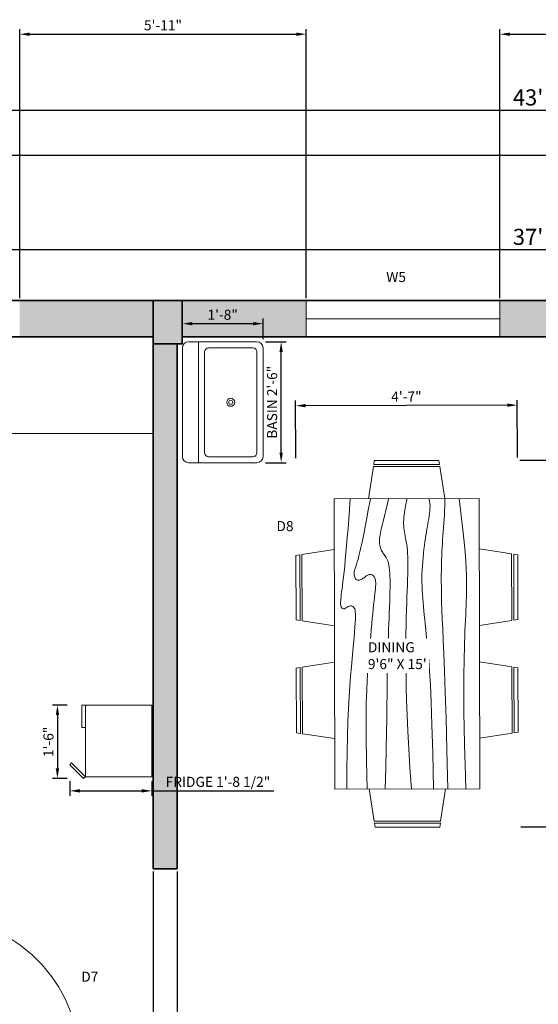
# Model space of a CAD drawing. Units: inches. Extents: x 5395 to 6469, y -203 to 448.
# Tile 4 of 7: x 5587 to 5715, y 204 to 448. Entities that reach past the tile are written whole.
import ezdxf

# ---------------------------------------------------------------- set-up
doc = ezdxf.new("R2010")
doc.units = ezdxf.units.IN
for name, color, linetype, lineweight in [('A-ANNO-DIMS', 2, 'Continuous', 18), ('A-ANNO-TEXT', 6, 'Continuous', 18), ('A-AREA-IDEN', 6, 'Continuous', 18), ('A-COLS', 7, 'Continuous', 35), ('A-COLS-PATT', 2, 'Continuous', 13), ('A-EQPM', 70, 'Continuous', 18), ('A-FLOR-CASE', 32, 'Continuous', 18), ('A-FLOR-FIXT', 70, 'Continuous', 18), ('A-GLAZ', 4, 'Continuous', 18), ('A-WALL', 7, 'Continuous', 35), ('A-WALL-PATT', 11, 'Continuous', 9), ('C-PROP', 7, 'Continuous', 25), ('door', 240, 'Continuous', 18), ('furniture', 70, 'Continuous', 18)]:
    doc.layers.add(name, color=color, linetype=linetype, lineweight=lineweight)
doc.styles.get("Standard").update_dxf_attribs({"font": 'arial.ttf'})
doc.dimstyles.new('ISO-25', dxfattribs={"dimtxt": 2.5, "dimasz": 2.5, "dimexe": 1.25, "dimexo": 0.625, "dimtad": 1, "dimdec": 1, "dimlunit": 3, "dimtxsty": 'Standard', "dimcen": 2.5, "dimadec": 0, "dimazin": 0, "dimtfac": 1, "dimtdec": 1, "dimtmove": 0, "dimatfit": 3, "dimfxl": 1, "dimarcsym": 0})

# ---------------------------------------------------------------- blocks, each defined once
blk = doc.blocks.new('*U4')
for p, q in [((0, 0), (0, 5)), ((30, 0), (30, 5))]:
    blk.add_line(p, q)
blk.add_lwpolyline([(0, 0), (0, -30), (1.75, -30), (1.75, 0)], close=True)
blk.add_arc((0, 0), 30, 270, 0)
blk = doc.blocks.new('Dining Set - 36 x 72 in.')
for p, q in [((-22, 27.5), (-22.1562, 26.50042)), ((-22, 27.5), (-6, 27.5)), ((-5.8437, 26.49966), (-6, 27.5)), ((6, 27.5), (5.8438, 26.50042)), ((6, 27.5), (22, 27.5)), ((22.1563, 26.49966), (22, 27.5)), ((-22.2343, 26.00059), (-23.4847, 17.99762)), ((-22.2304, 26), (-5.7608, 26)), ((-5.8416, 26.5), (-22.1534, 26.5)), ((-4.5152, 17.99762), (-5.7655, 25.99926)), ((5.7657, 26.00059), (4.5153, 17.99762)), ((5.7696, 26), (22.2392, 26)), ((22.1584, 26.5), (5.8466, 26.5)), ((23.4848, 17.99762), (22.2345, 25.99926)), ((36, 18), (-36, 18)), ((-36, 18), (-36, -18)), ((36, -18), (36, 18)), ((-45.5, 8), (-44.5004, 8.15617)), ((-45.5, 8), (-45.5, -8)), ((-44.5, -8.15843), (-44.5, 8.15338)), ((-44.0006, 8.23428), (-35.9976, 9.48474)), ((-44, 8.23041), (-44, -8.23915)), ((44.0006, 8.23428), (35.9976, 9.48474)), ((44, 8.23041), (44, -8.23915)), ((44.5, -8.15843), (44.5, 8.15338)), ((45.5, 8), (44.5005, 8.15617)), ((45.5, 8), (45.5, -8)), ((-44.4997, -8.15631), (-45.5, -8)), ((-35.9976, -9.48476), (-43.9993, -8.2345)), ((35.9976, -9.48476), (43.9993, -8.2345)), ((44.4997, -8.15631), (45.5, -8)), ((-36, -18), (36, -18)), ((-22.2343, -26.0006), (-23.4847, -17.99762)), ((-4.5152, -17.99762), (-5.7655, -25.99928)), ((5.7657, -26.0006), (4.5153, -17.99762)), ((23.4848, -17.99762), (22.2345, -25.99928)), ((-22.2304, -26), (-5.7608, -26)), ((-22, -27.5), (-22.1562, -26.50044)), ((-5.8416, -26.5), (-22.1534, -26.5)), ((-5.8437, -26.49967), (-6, -27.5)), ((5.7696, -26), (22.2392, -26)), ((6, -27.5), (5.8438, -26.50044)), ((22.1584, -26.5), (5.8466, -26.5)), ((22.1563, -26.49967), (22, -27.5)), ((-22, -27.5), (-6, -27.5)), ((6, -27.5), (22, -27.5))]:
    blk.add_line(p, q)
for points in [[(-36, 15), (-31.1772, 14.97754), (-26.8079, 14.91406), (-22.8538, 14.81543), (-19.276, 14.6875), (-16.0362, 14.53613), (-13.0957, 14.36718), (-10.4159, 14.18652), (-7.9583, 14), (-5.6904, 13.81315), (-3.6035, 13.63021), (-1.6954, 13.45508), (0.0365, 13.29166), (1.5945, 13.14388), (2.9811, 13.01562), (4.1988, 12.9108), (5.25, 12.83333), (6.1393, 12.78613), (6.8802, 12.76823), (7.4883, 12.77767), (7.9792, 12.8125), (8.3685, 12.87077), (8.6719, 12.95052), (8.9049, 13.0498), (9.0833, 13.16666), (9.2205, 13.29899), (9.3216, 13.44401), (9.3895, 13.59879), (9.4271, 13.76041), (9.4373, 13.92594), (9.4232, 14.09245), (9.3875, 14.257), (9.3333, 14.41666), (9.2638, 14.56917), (9.1836, 14.71484), (9.0975, 14.85465), (9.0104, 14.98958), (8.9272, 15.1206), (8.8529, 15.2487), (8.7922, 15.37483), (8.75, 15.5), (8.7305, 15.62467), (8.7344, 15.74739), (8.7617, 15.86621), (8.8125, 15.97916), (8.8867, 16.08431), (8.9844, 16.17968), (9.1055, 16.26334), (9.25, 16.33333), (9.4189, 16.38802), (9.6172, 16.42708), (9.8506, 16.45052), (10.125, 16.45833), (10.4463, 16.45052), (10.8203, 16.42708), (11.2529, 16.38802), (11.75, 16.33333), (12.3184, 16.26318), (12.9694, 16.17838), (13.7151, 16.07991), (14.5677, 15.96875), (15.5395, 15.84586), (16.6426, 15.71224), (17.8893, 15.56884), (19.2917, 15.41666), (20.859, 15.25667), (22.5879, 15.08984), (24.4721, 14.91715), (26.5052, 14.73958), (28.6809, 14.5581), (30.9929, 14.3737), (33.4347, 14.18733), (36, 14)], [(-36, 10), (-28.9766, 10.14274), (-23.1725, 10.20442), (-18.4241, 10.19775), (-14.5677, 10.13541), (-11.4399, 10.03011), (-8.877, 9.89453), (-6.7154, 9.74137), (-4.7917, 9.58333), (-2.9698, 9.43082), (-1.2246, 9.28515), (0.4415, 9.14534), (2.026, 9.01041), (3.5266, 8.87939), (4.9408, 8.7513), (6.266, 8.62516), (7.5, 8.5), (8.6411, 8.37549), (9.6914, 8.2539), (10.6538, 8.13818), (11.5312, 8.03125), (12.3267, 7.93603), (13.043, 7.85547), (13.6831, 7.79248), (14.25, 7.75), (14.7471, 7.7303), (15.1797, 7.73307), (15.5537, 7.75732), (15.875, 7.80208), (16.1494, 7.86637), (16.3828, 7.94922), (16.5811, 8.04964), (16.75, 8.16666), (16.8944, 8.29915), (17.0143, 8.44531), (17.1089, 8.60319), (17.1771, 8.77083), (17.218, 8.94629), (17.2305, 9.1276), (17.2137, 9.31282), (17.1667, 9.5), (17.0895, 9.6875), (16.987, 9.875), (16.8649, 10.0625), (16.7292, 10.25), (16.5856, 10.4375), (16.4401, 10.625), (16.2985, 10.8125), (16.1667, 11), (16.05, 11.18733), (15.9518, 11.3737), (15.8752, 11.5581), (15.8229, 11.73958), (15.798, 11.91715), (15.8034, 12.08984), (15.842, 12.25667), (15.9167, 12.41666), (16.0295, 12.56836), (16.1784, 12.70833), (16.3605, 12.83268), (16.5729, 12.9375), (16.8127, 13.01888), (17.0768, 13.07291), (17.3625, 13.0957), (17.6667, 13.08333), (17.9894, 13.03312), (18.3418, 12.94726), (18.7382, 12.82918), (19.1927, 12.68229), (19.7195, 12.51001), (20.3327, 12.31575), (21.0465, 12.10294), (21.875, 11.875), (22.8357, 11.63354), (23.959, 11.37304), (25.2786, 11.08618), (26.8282, 10.76562), (28.6414, 10.40405), (30.752, 9.99414), (33.1936, 9.52856), (36, 9)], [(-36, 5.5), (-30.7157, 5.3348), (-26.069, 5.20963), (-21.9946, 5.11767), (-18.4271, 5.05208), (-15.3009, 5.00602), (-12.5508, 4.97265), (-10.1112, 4.94515), (-7.9167, 4.91666), (-5.909, 4.88167), (-4.0586, 4.83984), (-2.3429, 4.79215), (-0.7396, 4.73958), (0.7739, 4.6831), (2.22, 4.6237), (3.6213, 4.56233), (5, 4.5), (6.373, 4.43782), (7.7344, 4.3776), (9.0723, 4.32129), (10.375, 4.27083), (11.6309, 4.22819), (12.8281, 4.19531), (13.9551, 4.17415), (15, 4.16666), (15.954, 4.17448), (16.819, 4.19791), (17.6001, 4.23698), (18.3021, 4.29166), (18.9299, 4.36198), (19.4883, 4.44791), (19.9823, 4.54948), (20.4167, 4.66666), (20.7969, 4.79899), (21.1302, 4.94401), (21.4245, 5.09879), (21.6875, 5.26041), (21.9271, 5.42594), (22.1511, 5.59245), (22.3672, 5.757), (22.5834, 5.91666), (22.8065, 6.06868), (23.0404, 6.21093), (23.2879, 6.34147), (23.5521, 6.45833), (23.8358, 6.55957), (24.142, 6.64323), (24.4735, 6.70735), (24.8334, 6.75), (25.2235, 6.76969), (25.642, 6.76692), (26.0858, 6.74267), (26.5521, 6.69791), (27.0379, 6.63362), (27.5404, 6.55078), (28.0565, 6.45036), (28.5834, 6.33333), (29.1242, 6.19987), (29.7071, 6.04687), (30.3661, 5.87044), (31.1354, 5.66666), (32.0493, 5.43164), (33.142, 5.16146), (34.4475, 4.85221), (36, 4.5)], [(-36, -1), (-30.7915, -0.6591), (-26.0195, -0.38216), (-21.6519, -0.16284), (-17.6563, 0.00521), (-14.0005, 0.12833), (-10.6523, 0.21289), (-7.5796, 0.26522), (-4.75, 0.29166), (-2.134, 0.29793), (0.2878, 0.28711), (2.5317, 0.26163), (4.6146, 0.22396), (6.5529, 0.17651), (8.3633, 0.12174), (10.0623, 0.06209), (11.6667, 0), (13.1899, -0.06201), (14.6341, -0.1211), (15.9982, -0.17432), (17.2813, -0.21875), (18.4823, -0.25147), (19.6003, -0.26953), (20.6343, -0.27002), (21.5834, -0.25), (22.4481, -0.20768), (23.2357, -0.14584), (23.9549, -0.06836), (24.6146, 0.02083), (25.2235, 0.11784), (25.7904, 0.21875), (26.3241, 0.31966), (26.8334, 0.41666), (27.3265, 0.50618), (27.8099, 0.58593), (28.2894, 0.65397), (28.7709, 0.70833), (29.2601, 0.74707), (29.763, 0.76823), (30.2855, 0.76985), (30.8334, 0.75), (31.4088, 0.70784), (31.9994, 0.64713), (32.589, 0.57275), (33.1615, 0.48958), (33.7008, 0.4025), (34.1908, 0.3164), (34.6153, 0.23616), (34.9584, 0.16666), (35.2099, 0.11165), (35.3848, 0.07031), (35.504, 0.04069), (35.5886, 0.02083), (35.6594, 0.00879), (35.7377, 0.0026), (35.8442, 0.00032), (36, 0)], [(-36, -6.5), (-27.1843, -6.31267), (-20.084, -6.1263), (-14.469, -5.9419), (-10.1094, -5.76042), (-6.7752, -5.58285), (-4.2363, -5.41016), (-2.2629, -5.24333), (-0.625, -5.08334), (0.8708, -4.93099), (2.2715, -4.78646), (3.5872, -4.64974), (4.8281, -4.52084), (6.0046, -4.39974), (7.127, -4.28646), (8.2053, -4.18099), (9.25, -4.08334), (10.2705, -3.99382), (11.2734, -3.91407), (12.2647, -3.84603), (13.25, -3.79167), (14.2354, -3.75293), (15.2266, -3.73177), (16.2295, -3.73015), (17.25, -3.75), (18.2912, -3.79248), (19.3451, -3.85547), (20.4009, -3.93604), (21.4479, -4.03125), (22.4754, -4.13819), (23.4727, -4.25391), (24.4289, -4.37549), (25.3334, -4.5), (26.1785, -4.62492), (26.9694, -4.74935), (27.7145, -4.87281), (28.4219, -4.99479), (29.1, -5.11483), (29.7572, -5.23242), (30.4016, -5.34709), (31.0417, -5.45834), (31.6837, -5.56437), (32.3262, -5.65821), (32.9658, -5.73153), (33.599, -5.77604), (34.2224, -5.78345), (34.8327, -5.74545), (35.4264, -5.65373), (36, -5.5)], [(-36, -10), (-26.4022, -9.81299), (-18.4675, -9.62891), (-11.9839, -9.45069), (-6.7396, -9.28125), (-2.5226, -9.12354), (0.8789, -8.98047), (3.6769, -8.85498), (6.0833, -8.75), (8.2767, -8.66765), (10.3021, -8.60677), (12.1712, -8.56543), (13.8958, -8.54167), (15.4876, -8.53353), (16.9583, -8.53907), (18.3197, -8.55632), (19.5834, -8.58334), (20.7616, -8.61841), (21.8685, -8.66081), (22.9188, -8.71004), (23.9271, -8.76563), (24.9081, -8.82707), (25.8763, -8.89388), (26.8465, -8.96558), (27.8334, -9.04167), (28.8474, -9.12118), (29.8828, -9.20117), (30.93, -9.27824), (31.9792, -9.34896), (33.0205, -9.40991), (34.0443, -9.45768), (35.0407, -9.48885), (36, -9.5)], [(-36, -14.5), (-30.0881, -14.33513), (-25.0332, -14.21224), (-20.7312, -14.12647), (-17.0781, -14.07292), (-13.97, -14.04671), (-11.3027, -14.04297), (-8.9724, -14.05681), (-6.875, -14.08334), (-4.9224, -14.11833), (-3.0905, -14.16016), (-1.3709, -14.20785), (0.2448, -14.26042), (1.7647, -14.3169), (3.1973, -14.3763), (4.5507, -14.43767), (5.8333, -14.5), (7.0554, -14.5621), (8.235, -14.62175), (9.3922, -14.67652), (10.5469, -14.72396), (11.7192, -14.76164), (12.929, -14.78711), (14.1965, -14.79794), (15.5417, -14.79167), (16.9933, -14.76424), (18.6152, -14.70508), (20.4804, -14.60197), (22.6615, -14.44271), (25.2312, -14.21509), (28.2624, -13.9069), (31.8277, -13.50594), (36, -13)]]:
    blk.add_lwpolyline(points)
blk = doc.blocks.new('Sink-single - 30 in top')
blk.add_line((-15, -3.999996), (15, -3.999996))
for points in [[(-13.5, 0), (13.5, 0)], [(-15, -18.499996), (-15, -1.5)], [(15, -1.5), (15, -18.499996)], [(-13.5, -17.499996), (-13.5, -6.499996)], [(-12.5, -5.499996), (12.5, -5.499996)], [(13.5, -6.499996), (13.5, -17.499996)], [(12.5, -18.499996), (-12.5, -18.499996)], [(13.5, -19.999996), (-13.5, -19.999996)]]:
    blk.add_lwpolyline(points)
for radius in [1, 0.5]:
    blk.add_circle((0, -11.999996), radius)
for centre, radius, start, end in [((-13.5, -1.5), 1.5, 90, 180), ((13.5, -1.5), 1.5, 0, 90), ((-12.5, -6.499996), 1, 90, 180), ((12.5, -6.499996), 1, 0, 90), ((-13.5, -18.499996), 1.5, 180, 270), ((-12.5, -17.499996), 1, 180, 270), ((12.5, -17.499996), 1, 270, 0), ((13.5, -18.499996), 1.5, 270, 0)]:
    blk.add_arc(centre, radius, start, end)
blk = doc.blocks.new('FRIDGE')
for points in [[(0, 16.47), (17.77, 16.47), (17.77, 0), (0, 0)], [(0, 0), (5.53, 0), (5.53, -0.88), (0, -0.88)], [(18.23, -0.47), (17.77, 0), (14.32, -3.43), (14.79, -3.9)]]:
    blk.add_lwpolyline(points, close=True)
blk = doc.blocks.new('*D17')
at = {"layer": 'A-ANNO-DIMS', "color": 0, "lineweight": -2, "transparency": 16777216}
for p, q in [((5490.94, 378.93), (5490.94, 392.2)), ((5493.44, 390.95), (5932.44, 390.95)), ((5934.94, 378.93), (5934.94, 392.2))]:
    blk.add_line(p, q, dxfattribs=at)
at = {"layer": 'A-ANNO-DIMS', "color": 0, "transparency": 16777216}
for points in [[(5493.44, 391.36), (5493.44, 390.53), (5490.94, 390.95)], [(5932.44, 391.36), (5932.44, 390.53), (5934.94, 390.95)]]:
    blk.add_solid(points, dxfattribs=at)
at = {"layer": 'Defpoints', "color": 0, "transparency": 16777216}
for p in [(5934.94, 390.95), (5490.94, 378.31), (5934.94, 378.31)]:
    blk.add_point(p, dxfattribs=at)
at = {"layer": 'A-ANNO-DIMS', "color": 0, "transparency": 16777216, "insert": (5712.94, 393.61), "char_height": 4, "attachment_point": 5}
blk.add_mtext("37'", dxfattribs=at)
blk = doc.blocks.new('*D18')
at = {"layer": 'A-ANNO-DIMS', "color": 0, "lineweight": -2, "transparency": 16777216}
for p, q in [((5454.94, 414.93), (5454.94, 426.78)), ((5457.44, 425.53), (5968.44, 425.53)), ((5970.94, 414.93), (5970.94, 426.78))]:
    blk.add_line(p, q, dxfattribs=at)
at = {"layer": 'A-ANNO-DIMS', "color": 0, "transparency": 16777216}
for points in [[(5457.44, 425.95), (5457.44, 425.12), (5454.94, 425.53)], [(5968.44, 425.95), (5968.44, 425.12), (5970.94, 425.53)]]:
    blk.add_solid(points, dxfattribs=at)
at = {"layer": 'Defpoints', "color": 0, "transparency": 16777216}
for p in [(5970.94, 425.53), (5454.94, 414.31), (5970.94, 414.31)]:
    blk.add_point(p, dxfattribs=at)
at = {"layer": 'A-ANNO-DIMS', "color": 0, "transparency": 16777216, "insert": (5712.94, 428.2), "char_height": 4, "attachment_point": 5}
blk.add_mtext("43'", dxfattribs=at)
blk = doc.blocks.new('WINDOW-48IN')
for p, q in [((0, 0), (0, 9)), ((48, 0), (48, 9)), ((0, 4.5), (48, 4.5))]:
    blk.add_line(p, q)
blk = doc.blocks.new('*D51')
at = {"layer": 'A-ANNO-DIMS', "color": 0, "lineweight": -2, "transparency": 16777216}
for p, q in [((5710.93, 338.72), (5725.21, 338.76)), ((5724.17, 250.25), (5723.96, 336.25)), ((5711.15, 247.72), (5725.43, 247.76))]:
    blk.add_line(p, q, dxfattribs=at)
at = {"layer": 'A-ANNO-DIMS', "color": 0, "transparency": 16777216}
for points in [[(5724.38, 336.25), (5723.55, 336.25), (5723.96, 338.75)], [(5724.59, 250.25), (5723.75, 250.25), (5724.18, 247.75)]]:
    blk.add_solid(points, dxfattribs=at)
at = {"layer": 'Defpoints', "color": 0, "transparency": 16777216}
for p in [(5710.31, 338.72), (5723.96, 338.75), (5710.53, 247.72)]:
    blk.add_point(p, dxfattribs=at)
at = {"layer": 'A-ANNO-DIMS', "color": 0, "transparency": 16777216, "insert": (5725.98, 293.26), "char_height": 2.5, "attachment_point": 5, "rotation": 270.1373}
blk.add_mtext('DINING SET 7\'-7"', dxfattribs=at)
blk = doc.blocks.new('*D52')
at = {"layer": 'A-ANNO-DIMS', "color": 0, "lineweight": -2, "transparency": 16777216}
for p, q in [((5655.31, 339.21), (5655.27, 353.49)), ((5707.77, 352.36), (5657.78, 352.24)), ((5710.31, 339.34), (5710.27, 353.62))]:
    blk.add_line(p, q, dxfattribs=at)
at = {"layer": 'A-ANNO-DIMS', "color": 0, "transparency": 16777216}
for points in [[(5657.77, 352.66), (5657.78, 351.83), (5655.28, 352.24)], [(5707.77, 352.78), (5707.78, 351.95), (5710.27, 352.37)]]:
    blk.add_solid(points, dxfattribs=at)
at = {"layer": 'Defpoints', "color": 0, "transparency": 16777216}
for p in [(5655.28, 352.24), (5655.31, 338.59), (5710.31, 338.72)]:
    blk.add_point(p, dxfattribs=at)
at = {"layer": 'A-ANNO-DIMS', "color": 0, "transparency": 16777216, "insert": (5682.77, 354.18), "char_height": 2.5, "attachment_point": 5, "rotation": 0.1373}
blk.add_mtext('4\'-7"', dxfattribs=at)
blk = doc.blocks.new('*D53')
at = {"layer": 'A-ANNO-DIMS', "color": 0, "lineweight": -2, "transparency": 16777216}
for p, q in [((5647.83, 368.08), (5652.96, 368.08)), ((5651.71, 340.58), (5651.71, 365.58)), ((5647.83, 338.08), (5652.96, 338.08))]:
    blk.add_line(p, q, dxfattribs=at)
at = {"layer": 'A-ANNO-DIMS', "color": 0, "transparency": 16777216}
for points in [[(5651.29, 365.58), (5652.12, 365.58), (5651.71, 368.08)], [(5651.29, 340.58), (5652.12, 340.58), (5651.71, 338.08)]]:
    blk.add_solid(points, dxfattribs=at)
at = {"layer": 'Defpoints', "color": 0, "transparency": 16777216}
for p in [(5647.21, 368.08), (5651.71, 368.08), (5647.21, 338.08)]:
    blk.add_point(p, dxfattribs=at)
at = {"layer": 'A-ANNO-DIMS', "color": 0, "transparency": 16777216, "insert": (5649.79, 353.08), "char_height": 2.5, "attachment_point": 5, "rotation": 90}
blk.add_mtext('BASIN 2\'-6"', dxfattribs=at)
blk = doc.blocks.new('*D54')
at = {"layer": 'A-ANNO-DIMS', "color": 0, "lineweight": -2, "transparency": 16777216}
for p, q in [((5627.21, 368.71), (5627.21, 373.83)), ((5647.21, 368.71), (5647.21, 373.83)), ((5644.71, 372.58), (5629.71, 372.58))]:
    blk.add_line(p, q, dxfattribs=at)
at = {"layer": 'A-ANNO-DIMS', "color": 0, "transparency": 16777216}
for points in [[(5629.71, 373), (5629.71, 372.17), (5627.21, 372.58)], [(5644.71, 373), (5644.71, 372.17), (5647.21, 372.58)]]:
    blk.add_solid(points, dxfattribs=at)
at = {"layer": 'Defpoints', "color": 0, "transparency": 16777216}
for p in [(5627.21, 372.58), (5627.21, 368.08), (5647.21, 368.08)]:
    blk.add_point(p, dxfattribs=at)
at = {"layer": 'A-ANNO-DIMS', "color": 0, "transparency": 16777216, "insert": (5637.21, 374.48), "char_height": 2.5, "attachment_point": 5}
blk.add_mtext('1\'-8"', dxfattribs=at)
blk = doc.blocks.new('*D55')
at = {"layer": 'A-ANNO-DIMS', "color": 0, "lineweight": -2, "transparency": 16777216}
for p, q in [((5599.29, 259.09), (5599.29, 255.41)), ((5619.66, 259.09), (5619.66, 255.41)), ((5601.79, 256.66), (5617.16, 256.66)), ((5619.66, 256.66), (5649.9, 256.66))]:
    blk.add_line(p, q, dxfattribs=at)
at = {"layer": 'A-ANNO-DIMS', "color": 0, "transparency": 16777216}
for points in [[(5601.79, 257.08), (5601.79, 256.25), (5599.29, 256.66)], [(5617.16, 257.08), (5617.16, 256.25), (5619.66, 256.66)]]:
    blk.add_solid(points, dxfattribs=at)
at = {"layer": 'Defpoints', "color": 0, "transparency": 16777216}
for p in [(5599.29, 259.72), (5619.66, 259.72), (5619.66, 256.66)]:
    blk.add_point(p, dxfattribs=at)
at = {"layer": 'A-ANNO-DIMS', "color": 0, "transparency": 16777216, "insert": (5636.03, 258.58), "char_height": 2.5, "attachment_point": 5}
blk.add_mtext('FRIDGE 1\'-8 1/2"', dxfattribs=at)
blk = doc.blocks.new('*D56')
at = {"layer": 'A-ANNO-DIMS', "color": 0, "lineweight": -2, "transparency": 16777216}
for p, q in [((5598.66, 277.95), (5594.98, 277.95)), ((5596.23, 275.45), (5596.23, 262.22)), ((5598.66, 259.72), (5594.98, 259.72))]:
    blk.add_line(p, q, dxfattribs=at)
at = {"layer": 'A-ANNO-DIMS', "color": 0, "transparency": 16777216}
for points in [[(5595.82, 275.45), (5596.65, 275.45), (5596.23, 277.95)], [(5595.82, 262.22), (5596.65, 262.22), (5596.23, 259.72)]]:
    blk.add_solid(points, dxfattribs=at)
at = {"layer": 'Defpoints', "color": 0, "transparency": 16777216}
for p in [(5599.29, 277.95), (5596.23, 259.72), (5599.29, 259.72)]:
    blk.add_point(p, dxfattribs=at)
at = {"layer": 'A-ANNO-DIMS', "color": 0, "transparency": 16777216, "insert": (5594.33, 268.83), "char_height": 2.5, "attachment_point": 5, "rotation": 90}
blk.add_mtext('1\'-6"', dxfattribs=at)
blk = doc.blocks.new('*D62')
at = {"layer": 'A-ANNO-DIMS', "color": 0, "lineweight": -2, "transparency": 16777216}
for p, q in [((5586.88, 378.93), (5586.88, 445.66)), ((5657.93, 378.93), (5657.93, 445.66)), ((5589.38, 444.41), (5655.43, 444.41))]:
    blk.add_line(p, q, dxfattribs=at)
at = {"layer": 'A-ANNO-DIMS', "color": 0, "transparency": 16777216}
for points in [[(5589.38, 444.82), (5589.38, 443.99), (5586.88, 444.41)], [(5655.43, 444.82), (5655.43, 443.99), (5657.93, 444.41)]]:
    blk.add_solid(points, dxfattribs=at)
at = {"layer": 'Defpoints', "color": 0, "transparency": 16777216}
for p in [(5657.93, 444.41), (5586.88, 378.31), (5657.93, 378.31)]:
    blk.add_point(p, dxfattribs=at)
at = {"layer": 'A-ANNO-DIMS', "color": 0, "transparency": 16777216, "insert": (5622.4, 446.31), "char_height": 2.5, "attachment_point": 5}
blk.add_mtext('5\'-11"', dxfattribs=at)
blk = doc.blocks.new('*D63')
at = {"layer": 'A-ANNO-DIMS', "color": 0, "lineweight": -2, "transparency": 16777216}
for p, q in [((5705.93, 378.93), (5705.93, 445.66)), ((5812.1, 378.93), (5812.1, 445.66)), ((5708.43, 444.41), (5809.6, 444.41))]:
    blk.add_line(p, q, dxfattribs=at)
at = {"layer": 'A-ANNO-DIMS', "color": 0, "transparency": 16777216}
for points in [[(5708.43, 444.82), (5708.43, 443.99), (5705.93, 444.41)], [(5809.6, 444.82), (5809.6, 443.99), (5812.1, 444.41)]]:
    blk.add_solid(points, dxfattribs=at)
at = {"layer": 'Defpoints', "color": 0, "transparency": 16777216}
for p in [(5812.1, 444.41), (5705.93, 378.31), (5812.1, 378.31)]:
    blk.add_point(p, dxfattribs=at)
at = {"layer": 'A-ANNO-DIMS', "color": 0, "transparency": 16777216, "insert": (5759.01, 446.31), "char_height": 2.5, "attachment_point": 5}
blk.add_mtext('8\'-10"', dxfattribs=at)
blk = doc.blocks.new('*D72')
at = {"layer": 'A-ANNO-DIMS', "color": 0, "lineweight": -2, "transparency": 16777216}
for p, q in [((5619.94, 236.68), (5619.94, -186.04)), ((5625.94, 236.68), (5625.94, -186.04)), ((5617.44, -184.79), (5614.94, -184.79)), ((5619.94, -184.79), (5625.94, -184.79)), ((5628.44, -184.79), (5638.83, -184.79))]:
    blk.add_line(p, q, dxfattribs=at)
at = {"layer": 'A-ANNO-DIMS', "color": 0, "transparency": 16777216}
for points in [[(5617.44, -184.38), (5617.44, -185.21), (5619.94, -184.79)], [(5628.44, -184.38), (5628.44, -185.21), (5625.94, -184.79)]]:
    blk.add_solid(points, dxfattribs=at)
at = {"layer": 'Defpoints', "color": 0, "transparency": 16777216}
for p in [(5619.94, 237.31), (5625.94, 237.31), (5625.94, -184.79)]:
    blk.add_point(p, dxfattribs=at)
at = {"layer": 'A-ANNO-DIMS', "color": 0, "transparency": 16777216, "insert": (5634.88, -182.89), "char_height": 2.5, "attachment_point": 5}
blk.add_mtext('0\'-6"', dxfattribs=at)

msp = doc.modelspace()

# ---------------------------------------------------------------- hatches: boundary and pattern name
at = {"layer": 'A-COLS-PATT'}
h = msp.add_hatch(color=256, dxfattribs=at)
h.dxf.hatch_style = 1
h.paths.add_polyline_path([(5627.19, 378.31), (5619.94, 378.31), (5619.94, 369.31), (5619.94, 367.55), (5627.19, 367.55), (5627.19, 369.31)])
h.paths.add_polyline_path([(5753.55, 378.31), (5739.94, 378.31), (5739.94, 369.31), (5753.55, 369.31)])
h.paths.add_polyline_path([(5934.94, 378.31), (5923.7, 378.31), (5923.7, 369.31), (5925.94, 369.31), (5934.94, 369.31)])
at = {"layer": 'A-WALL-PATT'}
h = msp.add_hatch(color=256, dxfattribs=at)
h.dxf.hatch_style = 1
h.paths.add_polyline_path([(5538.88, 378.31), (5499.94, 378.31), (5499.94, 369.31), (5538.88, 369.31)])
h.paths.add_polyline_path([(5499.94, 276.14), (5490.94, 276.14), (5490.94, 227.71), (5499.94, 227.71), (5499.94, 237.31)])
h.paths.add_polyline_path([(5565.94, 243.31), (5499.94, 243.31), (5499.94, 237.31), (5559.94, 237.31), (5559.94, 225.31), (5565.94, 225.31)])
h.paths.add_polyline_path([(5625.94, 367.55), (5619.94, 367.55), (5619.94, 237.31), (5625.94, 237.31)])
h.paths.add_polyline_path([(5745.94, 369.31), (5739.94, 369.31), (5739.94, 237.31), (5745.94, 237.31)])
h.paths.add_polyline_path([(5745.94, 192.25), (5739.94, 192.25), (5739.94, 190.23), (5745.94, 190.23)])
h.paths.add_polyline_path([(5745.94, 180.33), (5739.94, 180.33), (5739.94, 47.04), (5745.94, 47.04)])
h.paths.add_polyline_path([(5877.94, 183.31), (5884.03, 183.31), (5884.03, 189.31), (5747.34, 189.31), (5747.34, 183.31), (5871.94, 183.31), (5871.94, 82.27), (5877.94, 82.27), (5877.94, 90.31), (5925.94, 90.31), (5925.94, 96.31), (5877.94, 96.31)])
h.paths.add_polyline_path([(5934.94, 128.85), (5925.94, 128.85), (5925.94, 55.61), (5934.94, 55.61)])
h.paths.add_polyline_path([(5934.94, 181.4), (5925.94, 181.4), (5925.94, 152.85), (5934.94, 152.85)])
h.paths.add_polyline_path([(5925.94, 189.31), (5914.03, 189.31), (5914.03, 183.31), (5925.94, 183.31)], flags=17)
h.paths.add_polyline_path([(5934.94, 369.31), (5925.94, 369.31), (5925.94, 237.31), (5934.94, 237.31)])
h.paths.add_polyline_path([(5657.93, 378.31), (5627.19, 378.31), (5627.19, 369.31), (5657.93, 369.31)])
h.paths.add_polyline_path([(5619.94, 378.31), (5586.88, 378.31), (5586.88, 369.31), (5619.94, 369.31)])
h.paths.add_polyline_path([(5739.94, 378.31), (5705.93, 378.31), (5705.93, 369.31), (5739.94, 369.31)])
h.paths.add_polyline_path([(5812.1, 378.31), (5753.55, 378.31), (5753.55, 369.31), (5812.1, 369.31)])
h.paths.add_polyline_path([(5923.7, 378.31), (5860.1, 378.31), (5860.1, 369.31), (5923.7, 369.31)])
h.paths.add_polyline_path([(5499.94, 203.71), (5490.94, 203.71), (5490.94, 189.31), (5499.94, 189.31)])
h.paths.add_polyline_path([(5612.93, 189.31), (5499.94, 189.31), (5499.94, 183.31), (5612.93, 183.31)])
h.paths.add_polyline_path([(5499.94, 178.42), (5490.94, 178.42), (5490.94, 132.59), (5499.94, 132.59)])
h.paths.add_polyline_path([(5499.94, 84.59), (5490.94, 84.59), (5490.94, 47.04), (5499.94, 47.04)])
h.paths.add_polyline_path([(5499.94, 11.04), (5490.94, 11.04), (5490.94, 3.31), (5499.94, 3.31)])
h.paths.add_polyline_path([(5532.25, 3.31), (5502.78, 3.31), (5502.78, -5.69), (5532.25, -5.69)])
h.paths.add_polyline_path([(5601.84, 3.31), (5580.25, 3.31), (5580.25, -5.69), (5601.84, -5.69)])
h.paths.add_polyline_path([(5625.94, 3.31), (5614.13, 3.31), (5614.13, -5.69), (5625.94, -5.69)])
h.paths.add_polyline_path([(5787.9, 3.31), (5748.46, 3.31), (5748.46, -5.69), (5787.9, -5.69)])
h.paths.add_polyline_path([(5737.31, 3.31), (5697.94, 3.31), (5697.94, -5.69), (5737.31, -5.69)])
h.paths.add_polyline_path([(5745.94, 11.04), (5739.94, 11.04), (5739.94, 3.31), (5745.94, 3.31)])
h.paths.add_polyline_path([(5922.21, 3.31), (5877.94, 3.31), (5877.94, 46.27), (5871.94, 46.27), (5871.94, 3.31), (5835.9, 3.31), (5835.9, -5.69), (5922.21, -5.69)])
h.paths.add_polyline_path([(5934.94, 31.61), (5925.94, 31.61), (5925.94, 3.31), (5934.94, 3.31)])

# ---------------------------------------------------------------- linework, layer by layer
at = {"layer": 'A-COLS'}
for p, q in [((5619.94, 369.31), (5619.94, 378.31)), ((5627.19, 369.31), (5627.19, 378.31)), ((5627.19, 369.31), (5627.19, 367.55)), ((5619.94, 367.55), (5627.19, 367.55))]:
    msp.add_line(p, q, dxfattribs=at)
at = {"layer": 'A-FLOR-CASE'}
for points in [[(5499.94, 243.31), (5499.94, 369.31), (5619.94, 369.31)], [(5523.94, 243.31), (5523.94, 345.31), (5619.94, 345.31)]]:
    msp.add_lwpolyline(points, dxfattribs=at)
at = {"layer": 'A-WALL'}
for p, q in [((5490.94, 378.31), (5934.94, 378.31)), ((5490.94, 378.31), (5934.94, 378.31)), ((5934.94, 378.31), (5490.94, 378.31)), ((5499.94, 369.31), (5619.94, 369.31)), ((5619.94, 369.31), (5619.94, 237.31)), ((5619.94, 237.31), (5619.94, 369.31)), ((5627.19, 369.31), (5925.94, 369.31)), ((5625.94, 367.55), (5625.94, 237.31)), ((5619.94, 237.31), (5625.94, 237.31))]:
    msp.add_line(p, q, dxfattribs=at)
at = {"layer": 'C-PROP'}
msp.add_line((5934.94, 414.31), (5490.94, 414.31), dxfattribs=at)

# ---------------------------------------------------------------- block references
at = {"layer": 'A-EQPM', "rotation": 270}
msp.add_blockref('FRIDGE', (5603.19, 277.95), dxfattribs=at)
at = {"layer": 'A-FLOR-FIXT', "rotation": 90}
msp.add_blockref('Sink-single - 30 in top', (5627.21, 353.08), dxfattribs=at)
at = {"layer": 'A-GLAZ'}
msp.add_blockref('WINDOW-48IN', (5657.93, 369.31), dxfattribs=at)
at = {"layer": 'door', "xscale": 1.200014089153335, "yscale": 1.200014089153335, "zscale": 1.200014089153335, "rotation": 90}
msp.add_blockref('*U4', (5565.76, 189.31), dxfattribs=at)
at = {"layer": 'furniture', "rotation": 90.13732563059766}
msp.add_blockref('Dining Set - 36 x 72 in.', (5682.92, 293.15), dxfattribs=at)

# ---------------------------------------------------------------- texts
at = {"layer": 'A-ANNO-TEXT', "char_height": 2.5, "attachment_point": 1}
for s, insert in [('W5', (5677.77, 385.42)), ('D8', (5650.54, 323.61)), ('D7', (5602.14, 211.81))]:
    msp.add_mtext_dynamic_manual_height_columns(s, width=62.1492, gutter_width=12.5, heights=[0], dxfattribs=dict(at, insert=insert))

# ---------------------------------------------------------------- dimensions: what is measured, and where the dimension line sits
at = {"layer": 'A-ANNO-DIMS'}
for base, p1, p2, override, picture, middle in [((5657.9336, 444.405), (5586.8764, 378.305), (5657.9336, 378.305), {"dimdec": 1, "dimlfac": 1, "dimrnd": 0, "dimzin": 1, "dimdsep": 46, "dimlunit": 4, "dimfrac": 2}, '*D62', (5622.405, 446.3064)), ((5812.1, 444.41), (5705.93, 378.31), (5812.1, 378.31), {"dimdec": 1, "dimlfac": 1, "dimrnd": 0, "dimzin": 1, "dimdsep": 46, "dimlunit": 4, "dimfrac": 2}, '*D63', (5759.01, 446.31)), ((5934.94, 390.95), (5490.94, 378.31), (5934.94, 378.31), {"dimtxt": 4, "dimclrd": 0, "dimclre": 0, "dimclrt": 0}, '*D17', (5712.94, 393.61)), ((5625.94, -184.79), (5619.94, 237.31), (5625.94, 237.31), {"dimdec": 1, "dimlfac": 1, "dimrnd": 0, "dimzin": 1, "dimdsep": 46, "dimlunit": 4, "dimfrac": 2}, '*D72', (5634.88, -182.89))]:
    dim = msp.add_linear_dim(base=base, p1=p1, p2=p2, dimstyle='ISO-25', override=override, dxfattribs=at)
    dim.commit()
    dim.dimension.update_dxf_attribs({"geometry": picture, "text_midpoint": middle})
dim = msp.add_aligned_dim(p1=(5454.94, 414.31), p2=(5970.94, 414.31), distance=11.23, dimstyle='ISO-25', override={"dimtxt": 4, "dimclrd": 0, "dimclre": 0, "dimclrt": 0}, dxfattribs=at)
dim.commit()
dim.dimension.update_dxf_attribs({"geometry": '*D18', "text_midpoint": (5712.94, 428.2)})
for base, p1, p2, angle, picture, middle in [((5627.21, 372.58), (5647.21, 368.08), (5627.21, 368.08), 180, '*D54', (5637.21, 374.48)), ((5655.28, 352.24), (5710.31, 338.72), (5655.31, 338.59), 180.1373, '*D52', (5682.77, 354.18)), ((5596.23, 259.72), (5599.29, 277.95), (5599.29, 259.72), 270, '*D56', (5594.33, 268.83))]:
    dim = msp.add_linear_dim(base=base, p1=p1, p2=p2, angle=angle, dimstyle='ISO-25', override={"dimdec": 1, "dimlfac": 1, "dimrnd": 0, "dimzin": 1, "dimdsep": 46, "dimlunit": 4, "dimfrac": 2}, dxfattribs=at)
    dim.commit()
    dim.dimension.update_dxf_attribs({"geometry": picture, "text_midpoint": middle})
for base, p1, p2, angle, text, picture, middle in [((5651.71, 368.08), (5647.21, 338.08), (5647.21, 368.08), 90, 'BASIN <>', '*D53', (5649.79, 353.08)), ((5723.96, 338.75), (5710.53, 247.72), (5710.31, 338.72), 90.1373, 'DINING SET <>', '*D51', (5725.98, 293.26))]:
    dim = msp.add_linear_dim(base=base, p1=p1, p2=p2, angle=angle, text=text, dimstyle='ISO-25', override={"dimdec": 1, "dimlfac": 1, "dimrnd": 0, "dimzin": 1, "dimdsep": 46, "dimlunit": 4, "dimfrac": 2}, dxfattribs=at)
    dim.commit()
    dim.dimension.update_dxf_attribs({"geometry": picture, "text_midpoint": middle})
dim = msp.add_linear_dim(base=(5619.66, 256.66), p1=(5599.29, 259.72), p2=(5619.66, 259.72), text='FRIDGE <>', dimstyle='ISO-25', override={"dimdec": 1, "dimlfac": 1, "dimrnd": 0, "dimzin": 1, "dimdsep": 46, "dimlunit": 4, "dimfrac": 2}, dxfattribs=at)
dim.commit()
dim.dimension.update_dxf_attribs({"geometry": '*D55', "text_midpoint": (5636.03, 258.58)})

# ---------------------------------------------------------------- next in the draw order: wipeouts: each hides what was drawn before it
msp.add_wipeout([(5672.35, 285.91), (5688.4, 285.91), (5688.4, 294.42), (5672.35, 294.42)]).dxf.layer = 'A-AREA-IDEN'

# ---------------------------------------------------------------- next in the draw order: texts
at = {"layer": 'A-AREA-IDEN', "insert": (5673.22, 293.55), "char_height": 2.5, "width": 62.1492, "attachment_point": 1}
msp.add_mtext('DINING\\P9\'6" X 15\'', dxfattribs=at)

doc.saveas('drawing.dxf')
